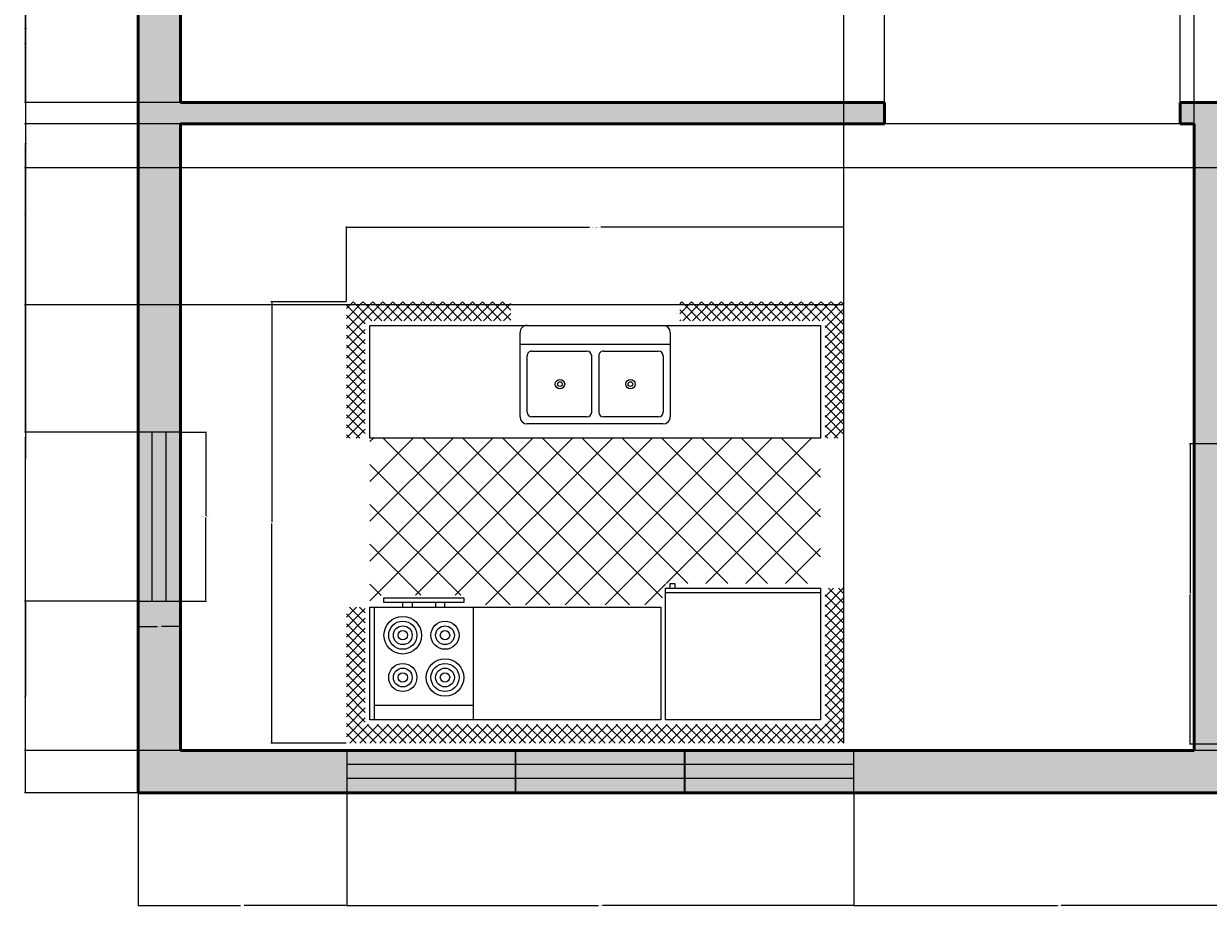
# Model space of a CAD drawing. Units: inches. Extents: x 1201 to 1754, y 247 to 775.
# Tile 1 of 10: x 1222 to 1475, y 247 to 435. Entities that reach past the tile are written whole.
import ezdxf

# ---------------------------------------------------------------- set-up
doc = ezdxf.new("R2010")
doc.units = ezdxf.units.IN
for name, color, linetype, lineweight in [('A-ANNO-DIMS', 2, 'Continuous', 18), ('A-FLOR-FIXT', 8, 'Continuous', 20), ('A-GLAZ', 4, 'Continuous', 18), ('A-GLAZ-PATT', 9, 'Continuous', 13), ('A-WALL', 7, 'Continuous', 50), ('A-WALL-PATT', 9, 'Continuous', 13)]:
    doc.layers.add(name, color=color, linetype=linetype, lineweight=lineweight)
doc.styles.get("Standard").update_dxf_attribs({"font": 'arial.ttf'})
doc.dimstyles.get("Standard").update_dxf_attribs({"dimtxt": 0.18, "dimasz": 0.18, "dimexe": 0.18, "dimexo": 0.0625, "dimgap": 0.09, "dimtad": 0, "dimtih": 1, "dimtoh": 1, "dimdec": 4, "dimzin": 0, "dimdsep": 46, "dimtxsty": 'Standard', "dimcen": 0.09, "dimadec": 0, "dimazin": 0, "dimtfac": 1, "dimtdec": 4, "dimtofl": 0, "dimtmove": 0, "dimatfit": 3, "dimfxl": 1, "dimtolj": 1, "dimtzin": 0, "dimarcsym": 0})

# ---------------------------------------------------------------- blocks, each defined once
blk = doc.blocks.new('Kitchen Layout - 7 x 8 ft')
for p, q in [((-5, 81.32), (2.68, 89)), ((-5, 83.44), (0.56, 89)), ((-5, 85.56), (-1.56, 89)), ((-5, 87.68), (-3.68, 89)), ((-1, 84.97), (-5, 88.97)), ((1.09, 85), (-2.91, 89)), ((3.21, 85), (-0.79, 89)), ((0.81, 85), (4.81, 89)), ((5.34, 85), (1.34, 89)), ((2.93, 85), (6.93, 89)), ((7.46, 85), (3.46, 89)), ((5.05, 85), (9.05, 89)), ((9.58, 85), (5.58, 89)), ((7.17, 85), (11.17, 89)), ((11.7, 85), (7.7, 89)), ((9.29, 85), (13.29, 89)), ((13.82, 85), (9.82, 89)), ((11.41, 85), (15.41, 89)), ((15.94, 85), (11.94, 89)), ((13.53, 85), (17.53, 89)), ((18.06, 85), (14.06, 89)), ((15.65, 85), (19.65, 89)), ((20.18, 85), (16.18, 89)), ((17.78, 85), (21.78, 89)), ((22.31, 85), (18.31, 89)), ((19.9, 85), (23.9, 89)), ((24.43, 85), (20.43, 89)), ((22.02, 85), (26.02, 89)), ((26.55, 85), (22.55, 89)), ((24.14, 85), (28.14, 89)), ((28.67, 85), (24.67, 89)), ((26.26, 85), (30.26, 89)), ((30.79, 85), (26.79, 89)), ((28.38, 85), (32.38, 89)), ((32.91, 85), (28.91, 89)), ((30.5, 85), (34.5, 89)), ((35.03, 85), (31.03, 89)), ((32.63, 85), (36.63, 89)), ((37.16, 85), (33.16, 89)), ((34.75, 85), (38.75, 89)), ((39.28, 85), (35.28, 89)), ((36.87, 85), (40.87, 89)), ((41.4, 85), (37.4, 89)), ((38.99, 85), (42.99, 89)), ((43.52, 85), (39.52, 89)), ((41.11, 85), (45.11, 89)), ((45.64, 85), (41.64, 89)), ((43.23, 85), (47.23, 89)), ((47.76, 85), (43.76, 89)), ((45.35, 85), (49.35, 89)), ((49.88, 85), (45.88, 89)), ((47.47, 85), (51.47, 89)), ((52, 85), (48, 89)), ((49.6, 85), (53.6, 89)), ((54.13, 85), (50.13, 89)), ((51.72, 85), (55.72, 89)), ((56.25, 85), (52.25, 89)), ((53.84, 85), (57.84, 89)), ((58.37, 85), (54.37, 89)), ((55.96, 85), (59.96, 89)), ((60.49, 85), (56.49, 89)), ((58.08, 85), (62.08, 89)), ((62.61, 85), (58.61, 89)), ((60.2, 85), (64.2, 89)), ((64.73, 85), (60.73, 89)), ((62.32, 85), (66.32, 89)), ((66.85, 85), (62.85, 89)), ((64.45, 85), (68.45, 89)), ((68.97, 85), (64.97, 89)), ((66.57, 85), (70.57, 89)), ((71.1, 85), (67.1, 89)), ((68.69, 85), (72.69, 89)), ((73.22, 85), (69.22, 89)), ((70.81, 85), (74.81, 89)), ((75.34, 85), (71.34, 89)), ((72.93, 85), (76.93, 89)), ((77.46, 85), (73.46, 89)), ((75.05, 85), (79.05, 89)), ((79.58, 85), (75.58, 89)), ((77.17, 85), (81.17, 89)), ((81.7, 85), (77.7, 89)), ((79.29, 85), (83.29, 89)), ((83.82, 85), (79.82, 89)), ((81.42, 85), (85.42, 89)), ((85.95, 85), (81.95, 89)), ((83.54, 85), (87.54, 89)), ((88.07, 85), (84.07, 89)), ((85.66, 85), (89.66, 89)), ((90.19, 85), (86.19, 89)), ((87.78, 85), (91.78, 89)), ((92.31, 85), (88.31, 89)), ((89.9, 85), (93.9, 89)), ((94.43, 85), (90.43, 89)), ((92.02, 85), (96.02, 89)), ((96.55, 85), (92.55, 89)), ((94.14, 85), (98.14, 89)), ((101, 82.67), (94.67, 89)), ((96.27, 85), (100.27, 89)), ((101, 84.79), (96.79, 89)), ((101, 86.92), (98.92, 89)), ((-1, 82.85), (-5, 86.85)), ((97, 83.61), (101, 87.61)), ((-1, 80.73), (-5, 84.73)), ((34, 84), (96, 84)), ((34, 60), (34, 84)), ((96, 84), (96, 60)), ((97, 81.49), (101, 85.49)), ((101, 80.55), (97, 84.55)), ((97, 79.37), (101, 83.37)), ((-5, 79.19), (-1, 83.19)), ((-1, 78.61), (-5, 82.61)), ((-5, 77.07), (-1, 81.07)), ((74, 81), (95, 81)), ((101, 78.43), (97, 82.43)), ((97, 77.25), (101, 81.25)), ((-1, 76.49), (-5, 80.49)), ((-5, 74.95), (-1, 78.95)), ((-1, 74.36), (-5, 78.36)), ((101, 76.31), (97, 80.31)), ((97, 75.13), (101, 79.13)), ((-5, 72.83), (-1, 76.83)), ((-1, 72.24), (-5, 76.24)), ((101, 74.19), (97, 78.19)), ((97, 73.01), (101, 77.01)), ((101, 72.07), (97, 76.07)), ((-5, 70.71), (-1, 74.71)), ((-1, 70.12), (-5, 74.12)), ((97, 70.89), (101, 74.89)), ((101, 69.95), (97, 73.95)), ((-5, 68.59), (-1, 72.59)), ((-1, 68), (-5, 72)), ((97, 68.76), (101, 72.76)), ((101, 67.82), (97, 71.82)), ((-5, 66.47), (-1, 70.47)), ((-1, 65.88), (-5, 69.88)), ((-5, 64.35), (-1, 68.35)), ((97, 66.64), (101, 70.64)), ((101, 65.7), (97, 69.7)), ((97, 64.52), (101, 68.52)), ((-1, 63.76), (-5, 67.76)), ((-5, 62.22), (-1, 66.22)), ((-1, 61.64), (-5, 65.64)), ((101, 63.58), (97, 67.58)), ((97, 62.4), (101, 66.4)), ((-5, 60.1), (-1, 64.1)), ((-1, 59.52), (-5, 63.52)), ((101, 61.46), (97, 65.46)), ((97, 60.28), (101, 64.28)), ((100.34, 60), (97, 63.34)), ((-5, 57.98), (-1, 61.98)), ((-1, 57.39), (-5, 61.39)), ((98.22, 60), (97, 61.22)), ((98.84, 60), (101, 62.16)), ((-1.73, 56), (-5, 59.27)), ((-4.86, 56), (-1, 59.86)), ((10.4, 24), (45.9, 59.5)), ((18.88, 24), (54.38, 59.5)), ((27.37, 24), (62.87, 59.5)), ((33.03, 55.11), (37.41, 59.5)), ((96, 60), (34, 60)), ((35.85, 24), (71.35, 59.5)), ((76.2, 24), (40.7, 59.5)), ((84.68, 24), (49.18, 59.5)), ((93.17, 24), (57.67, 59.5)), ((61.31, 24), (96, 58.69)), ((96, 29.65), (66.15, 59.5)), ((80, 60), (80, 59)), ((82, 59), (82, 60)), ((87, 59), (87, 60)), ((89, 60), (89, 59)), ((100.96, 60), (101, 60.04)), ((-3.85, 56), (-5, 57.15)), ((-2.74, 56), (-1, 57.74)), ((0, 57), (33, 57)), ((31, 55), (31, 56)), ((32, 56), (32, 55)), ((67.71, 24), (33.68, 58.04)), ((44.34, 24), (77.84, 57.5)), ((52.82, 24), (86.32, 57.5)), ((96, 38.14), (76.64, 57.5)), ((96, 46.63), (85.13, 57.5)), ((96, 55.11), (93.57, 57.54)), ((0, 30.57), (24.43, 55)), ((0, 39.06), (15.94, 55)), ((0, 47.54), (7.46, 55)), ((1.91, 24), (32.91, 55)), ((33.77, 24), (2.77, 55)), ((42.26, 24), (11.26, 55)), ((50.74, 24), (19.74, 55)), ((59.23, 24), (28.23, 55)), ((32, 55), (31, 55)), ((25.29, 24), (0, 49.29)), ((69.79, 24), (96, 50.21)), ((16.8, 24), (0, 40.8)), ((78.28, 24), (96, 41.72)), ((86.76, 24), (96, 33.24)), ((8.32, 24), (0, 32.32)), ((-5, 21.92), (-2.92, 24)), ((-5, 19.8), (-1, 23.8)), ((-1, 19.21), (-5, 23.21)), ((-1, 21.33), (-3.67, 24)), ((-1, 23.45), (-1.55, 24)), ((0, 24), (96, 24)), ((0, 0), (0, 24)), ((95.25, 24), (96, 24.75)), ((96, 24), (96, 0)), ((97, 22.1), (98.9, 24)), ((97, 19.97), (101, 23.97)), ((101, 19.03), (97, 23.03)), ((101, 21.16), (98.16, 24)), ((101, 23.28), (100.28, 24)), ((-5, 17.68), (-1, 21.68)), ((-1, 17.09), (-5, 21.09)), ((97, 17.85), (101, 21.85)), ((101, 16.91), (97, 20.91)), ((-5, 15.55), (-1, 19.55)), ((-1, 14.97), (-5, 18.97)), ((47.25, 6.5), (47.25, 18.5)), ((48.75, 18.5), (48.75, 6.5)), ((97, 15.73), (101, 19.73)), ((101, 14.79), (97, 18.79)), ((-5, 13.43), (-1, 17.43)), ((-1, 12.85), (-5, 16.85)), ((-5, 11.31), (-1, 15.31)), ((97, 13.61), (101, 17.61)), ((101, 12.67), (97, 16.67)), ((97, 11.49), (101, 15.49)), ((-1, 10.73), (-5, 14.73)), ((-5, 9.19), (-1, 13.19)), ((101, 10.55), (97, 14.55)), ((97, 9.37), (101, 13.37)), ((-1, 8.6), (-5, 12.6)), ((-5, 7.07), (-1, 11.07)), ((-1, 6.48), (-5, 10.48)), ((101, 8.43), (97, 12.43)), ((97, 7.25), (101, 11.25)), ((101, 6.31), (97, 10.31)), ((-5, 4.95), (-1, 8.95)), ((-1, 4.36), (-5, 8.36)), ((97, 5.12), (101, 9.12)), ((101, 4.18), (97, 8.18)), ((-5, 2.83), (-1, 6.83)), ((-1, 2.24), (-5, 6.24)), ((97, 3), (101, 7)), ((101, 2.06), (97, 6.06)), ((-5, 0.71), (-1, 4.71)), ((-1, 0.12), (-5, 4.12)), ((-5, -1.42), (-1, 2.58)), ((64, 4), (32, 4)), ((93.24, -5), (101, 2.76)), ((97, 0.88), (101, 4.88)), ((101, -0.06), (97, 3.94)), ((2, -5), (-5, 2)), ((-5, -3.54), (-1, 0.46)), ((96, 0), (0, 0)), ((95.36, -5), (101, 0.64)), ((101, -2.18), (97, 1.82)), ((-0.12, -5), (-5, -0.12)), ((-2.25, -5), (-5, -2.25)), ((-4.34, -5), (-0.34, -1)), ((-2.22, -5), (1.78, -1)), ((-0.1, -5), (3.9, -1)), ((4.12, -5), (0.12, -1)), ((2.02, -5), (6.02, -1)), ((6.24, -5), (2.24, -1)), ((4.14, -5), (8.14, -1)), ((8.36, -5), (4.36, -1)), ((6.27, -5), (10.27, -1)), ((10.48, -5), (6.48, -1)), ((8.39, -5), (12.39, -1)), ((12.6, -5), (8.6, -1)), ((10.51, -5), (14.51, -1)), ((14.73, -5), (10.73, -1)), ((12.63, -5), (16.63, -1)), ((16.85, -5), (12.85, -1)), ((14.75, -5), (18.75, -1)), ((18.97, -5), (14.97, -1)), ((16.87, -5), (20.87, -1)), ((21.09, -5), (17.09, -1)), ((18.99, -5), (22.99, -1)), ((23.21, -5), (19.21, -1)), ((21.11, -5), (25.11, -1)), ((25.33, -5), (21.33, -1)), ((23.24, -5), (27.24, -1)), ((27.45, -5), (23.45, -1)), ((25.36, -5), (29.36, -1)), ((29.57, -5), (25.57, -1)), ((27.48, -5), (30, -2.48)), ((30, -3.3), (27.7, -1)), ((30, -1.18), (29.82, -1)), ((66, -2.54), (67.54, -1)), ((66, -4.66), (69.66, -1)), ((69.88, -5), (66, -1.12)), ((67.78, -5), (71.78, -1)), ((72, -5), (68, -1)), ((69.9, -5), (73.9, -1)), ((74.12, -5), (70.12, -1)), ((72.03, -5), (76.03, -1)), ((76.24, -5), (72.24, -1)), ((74.15, -5), (78.15, -1)), ((78.36, -5), (74.36, -1)), ((76.27, -5), (80.27, -1)), ((80.49, -5), (76.49, -1)), ((78.39, -5), (82.39, -1)), ((82.61, -5), (78.61, -1)), ((80.51, -5), (84.51, -1)), ((84.73, -5), (80.73, -1)), ((82.63, -5), (86.63, -1)), ((86.85, -5), (82.85, -1)), ((84.75, -5), (88.75, -1)), ((88.97, -5), (84.97, -1)), ((86.88, -5), (90.88, -1)), ((91.09, -5), (87.09, -1)), ((89, -5), (93, -1)), ((93.21, -5), (89.21, -1)), ((91.12, -5), (95.12, -1)), ((95.34, -5), (91.34, -1)), ((97.46, -5), (93.46, -1)), ((99.58, -5), (95.58, -1)), ((101, -4.3), (97, -0.3)), ((97.48, -5), (101, -1.48)), ((-4.37, -5), (-5, -4.37)), ((29.6, -5), (30, -4.6)), ((67.76, -5), (66, -3.24)), ((99.6, -5), (101, -3.6))]:
    blk.add_line(p, q)
for points in [[(0, 56), (0, 84), (33, 84), (33, 56)], [(74, 60), (74, 84), (95, 84), (95, 60)], [(76, 58), (76, 59), (93, 59), (93, 58)]]:
    blk.add_lwpolyline(points, close=True)
for points in [[(33.5, 21), (62.5, 21)], [(32, 1.5), (32, 19.5)], [(33.5, 6.5), (33.5, 18.5)], [(34.5, 19.5), (46.25, 19.5)], [(49.75, 19.5), (61.5, 19.5)], [(62.5, 18.5), (62.5, 6.5)], [(64, 19.5), (64, 1.5)], [(46.25, 5.5), (34.5, 5.5)], [(61.5, 5.5), (49.75, 5.5)], [(62.5, 0), (33.5, 0)]]:
    blk.add_lwpolyline(points)
for centre, radius in [((80, 75), 4), ((80, 75), 3), ((80, 75), 2), ((80, 75), 1), ((89, 75), 3), ((89, 75), 2), ((89, 75), 1), ((80, 66), 3), ((89, 66), 4), ((89, 66), 3), ((80, 66), 2), ((80, 66), 1), ((89, 66), 2), ((89, 66), 1), ((40.5, 12.5), 1), ((40.5, 12.5), 0.5), ((55.5, 12.5), 1), ((55.5, 12.5), 0.5)]:
    blk.add_circle(centre, radius)
for centre, radius, start, end in [((33.5, 19.5), 1.5, 90, 180), ((62.5, 19.5), 1.5, 0, 90), ((34.5, 18.5), 1, 90, 180), ((46.25, 18.5), 1, 0, 90), ((49.75, 18.5), 1, 90, 180), ((61.5, 18.5), 1, 0, 90), ((34.5, 6.5), 1, 180, 270), ((46.25, 6.5), 1, 270, 0), ((49.75, 6.5), 1, 180, 270), ((61.5, 6.5), 1, 270, 0), ((33.5, 1.5), 1.5, 180, 270), ((62.5, 1.5), 1.5, 270, 0)]:
    blk.add_arc(centre, radius, start, end)
blk = doc.blocks.new('WIN-36IN-PLAN')
for p, q in [((9, 36), (0, 36)), ((3, 0), (3, 36)), ((6, 0), (6, 36))]:
    blk.add_line(p, q)
blk.add_lwpolyline([(0, 36), (0, 0), (9, 0), (9, 36)])
blk = doc.blocks.new('*D19')
at = {"layer": 'A-ANNO-DIMS', "color": 0, "lineweight": -2, "transparency": 16777216}
for p, q in [((1255.58, 347.75), (1261.1, 347.75)), ((1260.92, 347.57), (1260.92, 329.93)), ((1260.92, 311.93), (1260.92, 329.57)), ((1255.58, 311.75), (1261.1, 311.75))]:
    blk.add_line(p, q, dxfattribs=at)
at = {"layer": 'A-ANNO-DIMS', "color": 0, "transparency": 16777216}
for points in [[(1260.89, 347.57), (1260.95, 347.57), (1260.92, 347.75)], [(1260.89, 311.93), (1260.95, 311.93), (1260.92, 311.75)]]:
    blk.add_solid(points, dxfattribs=at)
at = {"layer": 'Defpoints', "color": 0, "transparency": 16777216}
for p in [(1255.52, 347.75), (1260.92, 347.75), (1255.52, 311.75)]:
    blk.add_point(p, dxfattribs=at)
at = {"layer": 'A-ANNO-DIMS', "color": 0, "transparency": 16777216, "insert": (1260.92, 329.75), "char_height": 0.18, "attachment_point": 5}
blk.add_mtext('\\A1;WINDOW 36 TYP.', dxfattribs=at)
blk = doc.blocks.new('*D20')
at = {"layer": 'A-ANNO-DIMS', "color": 0, "lineweight": -2, "transparency": 16777216}
for p, q in [((1246.52, 311.69), (1246.52, 306.17)), ((1255.52, 311.69), (1255.52, 306.17)), ((1246.7, 306.35), (1250.56, 306.35)), ((1255.34, 306.35), (1251.48, 306.35))]:
    blk.add_line(p, q, dxfattribs=at)
at = {"layer": 'A-ANNO-DIMS', "color": 0, "transparency": 16777216}
for points in [[(1246.7, 306.38), (1246.7, 306.32), (1246.52, 306.35)], [(1255.34, 306.38), (1255.34, 306.32), (1255.52, 306.35)]]:
    blk.add_solid(points, dxfattribs=at)
at = {"layer": 'Defpoints', "color": 0, "transparency": 16777216}
for p in [(1246.52, 311.75), (1255.52, 311.75), (1255.52, 306.35)]:
    blk.add_point(p, dxfattribs=at)
at = {"layer": 'A-ANNO-DIMS', "color": 0, "transparency": 16777216, "insert": (1251.02, 306.35), "char_height": 0.18, "attachment_point": 5}
blk.add_mtext('\\A1;9 TYP.', dxfattribs=at)
blk = doc.blocks.new('*D39')
at = {"layer": 'A-ANNO-DIMS', "color": 0, "lineweight": -2, "transparency": 16777216}
for p, q in [((1290.89, 375.55), (1290.89, 391.57)), ((1291.07, 391.39), (1342.69, 391.39)), ((1396.71, 391.39), (1345.09, 391.39)), ((1396.89, 375.55), (1396.89, 391.57))]:
    blk.add_line(p, q, dxfattribs=at)
at = {"layer": 'A-ANNO-DIMS', "color": 0, "transparency": 16777216}
for points in [[(1291.07, 391.42), (1291.07, 391.36), (1290.89, 391.39)], [(1396.71, 391.42), (1396.71, 391.36), (1396.89, 391.39)]]:
    blk.add_solid(points, dxfattribs=at)
at = {"layer": 'Defpoints', "color": 0, "transparency": 16777216}
for p in [(1290.89, 391.39), (1290.89, 375.49), (1396.89, 375.49)]:
    blk.add_point(p, dxfattribs=at)
at = {"layer": 'A-ANNO-DIMS', "color": 0, "transparency": 16777216, "insert": (1343.89, 391.39), "char_height": 0.18, "attachment_point": 5}
blk.add_mtext('\\A1;KITCHEN UNIT 106', dxfattribs=at)
blk = doc.blocks.new('*D40')
at = {"layer": 'A-ANNO-DIMS', "color": 0, "lineweight": -2, "transparency": 16777216}
for p, q in [((1290.83, 375.49), (1274.81, 375.49)), ((1274.99, 375.31), (1274.99, 328.67)), ((1274.99, 281.67), (1274.99, 328.31)), ((1290.83, 281.49), (1274.81, 281.49))]:
    blk.add_line(p, q, dxfattribs=at)
at = {"layer": 'A-ANNO-DIMS', "color": 0, "transparency": 16777216}
for points in [[(1274.96, 375.31), (1275.02, 375.31), (1274.99, 375.49)], [(1274.96, 281.67), (1275.02, 281.67), (1274.99, 281.49)]]:
    blk.add_solid(points, dxfattribs=at)
at = {"layer": 'Defpoints', "color": 0, "transparency": 16777216}
for p in [(1290.89, 375.49), (1274.99, 281.49), (1290.89, 281.49)]:
    blk.add_point(p, dxfattribs=at)
at = {"layer": 'A-ANNO-DIMS', "color": 0, "transparency": 16777216, "insert": (1274.99, 328.49), "char_height": 0.18, "attachment_point": 5}
blk.add_mtext('\\A1;94', dxfattribs=at)
blk = doc.blocks.new('*D43')
at = {"layer": 'A-ANNO-DIMS', "color": 0, "lineweight": -2, "transparency": 16777216}
for p, q in [((1480.23, 345.28), (1470.51, 345.28)), ((1470.69, 345.1), (1470.69, 313.47)), ((1470.69, 281.46), (1470.69, 313.1)), ((1480.23, 281.28), (1470.51, 281.28))]:
    blk.add_line(p, q, dxfattribs=at)
at = {"layer": 'A-ANNO-DIMS', "color": 0, "transparency": 16777216}
for points in [[(1470.66, 345.1), (1470.72, 345.1), (1470.69, 345.28)], [(1470.66, 281.46), (1470.72, 281.46), (1470.69, 281.28)]]:
    blk.add_solid(points, dxfattribs=at)
at = {"layer": 'Defpoints', "color": 0, "transparency": 16777216}
for p in [(1480.29, 345.28), (1470.69, 281.28), (1480.29, 281.28)]:
    blk.add_point(p, dxfattribs=at)
at = {"layer": 'A-ANNO-DIMS', "color": 0, "transparency": 16777216, "insert": (1470.69, 313.28), "char_height": 0.18, "attachment_point": 5}
blk.add_mtext('\\A1;REFRIGERATOR 64', dxfattribs=at)
blk = doc.blocks.new('*D50')
at = {"layer": 'A-ANNO-DIMS', "color": 0, "lineweight": -2, "transparency": 16777216}
for p, q in [((1255.46, 557.44), (1222.33, 557.44)), ((1222.51, 557.26), (1222.51, 487.87)), ((1222.51, 418.12), (1222.51, 487.51)), ((1255.46, 417.94), (1222.33, 417.94))]:
    blk.add_line(p, q, dxfattribs=at)
at = {"layer": 'A-ANNO-DIMS', "color": 0, "transparency": 16777216}
for points in [[(1222.48, 557.26), (1222.54, 557.26), (1222.51, 557.44)], [(1222.48, 418.12), (1222.54, 418.12), (1222.51, 417.94)]]:
    blk.add_solid(points, dxfattribs=at)
at = {"layer": 'Defpoints', "color": 0, "transparency": 16777216}
for p in [(1255.52, 557.44), (1222.51, 417.94), (1255.52, 417.94)]:
    blk.add_point(p, dxfattribs=at)
at = {"layer": 'A-ANNO-DIMS', "color": 0, "transparency": 16777216, "insert": (1222.51, 487.69), "char_height": 0.18, "attachment_point": 5}
blk.add_mtext('\\A1;139.5', dxfattribs=at)
blk = doc.blocks.new('*D51')
at = {"layer": 'A-ANNO-DIMS', "color": 0, "lineweight": -2, "transparency": 16777216}
for p, q in [((1471.46, 413.44), (1222.33, 413.44)), ((1222.51, 413.26), (1222.51, 346.87)), ((1222.51, 280.12), (1222.51, 346.51)), ((1471.46, 279.94), (1222.33, 279.94))]:
    blk.add_line(p, q, dxfattribs=at)
at = {"layer": 'A-ANNO-DIMS', "color": 0, "transparency": 16777216}
for points in [[(1222.48, 413.26), (1222.54, 413.26), (1222.51, 413.44)], [(1222.48, 280.12), (1222.54, 280.12), (1222.51, 279.94)]]:
    blk.add_solid(points, dxfattribs=at)
at = {"layer": 'Defpoints', "color": 0, "transparency": 16777216}
for p in [(1471.52, 413.44), (1222.51, 279.94), (1471.52, 279.94)]:
    blk.add_point(p, dxfattribs=at)
at = {"layer": 'A-ANNO-DIMS', "color": 0, "transparency": 16777216, "insert": (1222.51, 346.69), "char_height": 0.18, "attachment_point": 5}
blk.add_mtext('\\A1;133.5', dxfattribs=at)
blk = doc.blocks.new('*D58')
at = {"layer": 'A-ANNO-DIMS', "color": 0, "lineweight": -2, "transparency": 16777216}
for p, q in [((1405.52, 418), (1405.52, 775.14)), ((1405.7, 774.96), (1436.8, 774.96)), ((1468.34, 774.96), (1437.24, 774.96)), ((1468.52, 418), (1468.52, 775.14))]:
    blk.add_line(p, q, dxfattribs=at)
at = {"layer": 'A-ANNO-DIMS', "color": 0, "transparency": 16777216}
for points in [[(1405.7, 774.99), (1405.7, 774.93), (1405.52, 774.96)], [(1468.34, 774.99), (1468.34, 774.93), (1468.52, 774.96)]]:
    blk.add_solid(points, dxfattribs=at)
at = {"layer": 'Defpoints', "color": 0, "transparency": 16777216}
for p in [(1468.52, 774.96), (1405.52, 417.94), (1468.52, 417.94)]:
    blk.add_point(p, dxfattribs=at)
at = {"layer": 'A-ANNO-DIMS', "color": 0, "transparency": 16777216, "insert": (1437.02, 774.96), "char_height": 0.18, "attachment_point": 5}
blk.add_mtext('\\A1;63', dxfattribs=at)
blk = doc.blocks.new('*D59')
at = {"layer": 'A-ANNO-DIMS', "color": 0, "lineweight": -2, "transparency": 16777216}
for p, q in [((1255.52, 418), (1255.52, 775.14)), ((1255.7, 774.96), (1330.24, 774.96)), ((1405.34, 774.96), (1330.8, 774.96)), ((1405.52, 418), (1405.52, 775.14))]:
    blk.add_line(p, q, dxfattribs=at)
at = {"layer": 'A-ANNO-DIMS', "color": 0, "transparency": 16777216}
for points in [[(1255.7, 774.99), (1255.7, 774.93), (1255.52, 774.96)], [(1405.34, 774.99), (1405.34, 774.93), (1405.52, 774.96)]]:
    blk.add_solid(points, dxfattribs=at)
at = {"layer": 'Defpoints', "color": 0, "transparency": 16777216}
for p in [(1405.52, 774.96), (1255.52, 417.94), (1405.52, 417.94)]:
    blk.add_point(p, dxfattribs=at)
at = {"layer": 'A-ANNO-DIMS', "color": 0, "transparency": 16777216, "insert": (1330.52, 774.96), "char_height": 0.18, "attachment_point": 5}
blk.add_mtext('\\A1;150', dxfattribs=at)
blk = doc.blocks.new('*D69')
at = {"layer": 'A-ANNO-DIMS', "color": 0, "lineweight": -2, "transparency": 16777216}
for p, q in [((1246.46, 311.75), (1222.33, 311.75)), ((1222.51, 311.57), (1222.51, 291.53)), ((1222.51, 271.12), (1222.51, 291.16)), ((1246.46, 270.94), (1222.33, 270.94))]:
    blk.add_line(p, q, dxfattribs=at)
at = {"layer": 'A-ANNO-DIMS', "color": 0, "transparency": 16777216}
for points in [[(1222.48, 311.57), (1222.54, 311.57), (1222.51, 311.75)], [(1222.48, 271.12), (1222.54, 271.12), (1222.51, 270.94)]]:
    blk.add_solid(points, dxfattribs=at)
at = {"layer": 'Defpoints', "color": 0, "transparency": 16777216}
for p in [(1222.51, 311.75), (1246.52, 311.75), (1246.52, 270.94)]:
    blk.add_point(p, dxfattribs=at)
at = {"layer": 'A-ANNO-DIMS', "color": 0, "transparency": 16777216, "insert": (1222.51, 291.35), "char_height": 0.18, "attachment_point": 5}
blk.add_mtext('\\A1;40.81', dxfattribs=at)
blk = doc.blocks.new('*D70')
at = {"layer": 'A-ANNO-DIMS', "color": 0, "lineweight": -2, "transparency": 16777216}
for p, q in [((1246.46, 470.7), (1222.33, 470.7)), ((1222.51, 470.52), (1222.51, 409.4)), ((1222.51, 347.93), (1222.51, 409.04)), ((1246.46, 347.75), (1222.33, 347.75))]:
    blk.add_line(p, q, dxfattribs=at)
at = {"layer": 'A-ANNO-DIMS', "color": 0, "transparency": 16777216}
for points in [[(1222.48, 470.52), (1222.54, 470.52), (1222.51, 470.7)], [(1222.48, 347.93), (1222.54, 347.93), (1222.51, 347.75)]]:
    blk.add_solid(points, dxfattribs=at)
at = {"layer": 'Defpoints', "color": 0, "transparency": 16777216}
for p in [(1222.51, 470.7), (1246.52, 470.7), (1246.52, 347.75)]:
    blk.add_point(p, dxfattribs=at)
at = {"layer": 'A-ANNO-DIMS', "color": 0, "transparency": 16777216, "insert": (1222.51, 409.22), "char_height": 0.18, "attachment_point": 5}
blk.add_mtext('\\A1;122.95', dxfattribs=at)
blk = doc.blocks.new('*D74')
at = {"layer": 'A-ANNO-DIMS', "color": 0, "lineweight": -2, "transparency": 16777216}
for p, q in [((1717.46, 404.03), (1222.33, 404.03)), ((1222.51, 403.85), (1222.51, 342.17)), ((1222.51, 280.12), (1222.51, 341.81)), ((1717.46, 279.94), (1222.33, 279.94))]:
    blk.add_line(p, q, dxfattribs=at)
at = {"layer": 'A-ANNO-DIMS', "color": 0, "transparency": 16777216}
for points in [[(1222.48, 403.85), (1222.54, 403.85), (1222.51, 404.03)], [(1222.48, 280.12), (1222.54, 280.12), (1222.51, 279.94)]]:
    blk.add_solid(points, dxfattribs=at)
at = {"layer": 'Defpoints', "color": 0, "transparency": 16777216}
for p in [(1222.51, 404.03), (1717.52, 404.03), (1717.52, 279.94)]:
    blk.add_point(p, dxfattribs=at)
at = {"layer": 'A-ANNO-DIMS', "color": 0, "transparency": 16777216, "insert": (1222.51, 341.99), "char_height": 0.18, "attachment_point": 5}
blk.add_mtext('\\A1;124.1', dxfattribs=at)
blk = doc.blocks.new('*D77')
at = {"layer": 'A-ANNO-DIMS', "color": 0, "lineweight": -2, "transparency": 16777216}
for p, q in [((1246.52, 270.88), (1246.52, 246.75)), ((1290.95, 270.88), (1290.95, 246.75)), ((1246.7, 246.93), (1268.34, 246.93)), ((1290.77, 246.93), (1269.13, 246.93))]:
    blk.add_line(p, q, dxfattribs=at)
at = {"layer": 'A-ANNO-DIMS', "color": 0, "transparency": 16777216}
for points in [[(1246.7, 246.96), (1246.7, 246.9), (1246.52, 246.93)], [(1290.77, 246.96), (1290.77, 246.9), (1290.95, 246.93)]]:
    blk.add_solid(points, dxfattribs=at)
at = {"layer": 'Defpoints', "color": 0, "transparency": 16777216}
for p in [(1246.52, 270.94), (1290.95, 270.94), (1290.95, 246.93)]:
    blk.add_point(p, dxfattribs=at)
at = {"layer": 'A-ANNO-DIMS', "color": 0, "transparency": 16777216, "insert": (1268.73, 246.93), "char_height": 0.18, "attachment_point": 5}
blk.add_mtext('\\A1;44.43', dxfattribs=at)
blk = doc.blocks.new('*D78')
at = {"layer": 'A-ANNO-DIMS', "color": 0, "lineweight": -2, "transparency": 16777216}
for p, q in [((1290.95, 270.88), (1290.95, 246.75)), ((1399.01, 270.88), (1399.01, 246.75)), ((1291.13, 246.93), (1344.52, 246.93)), ((1398.83, 246.93), (1345.43, 246.93))]:
    blk.add_line(p, q, dxfattribs=at)
at = {"layer": 'A-ANNO-DIMS', "color": 0, "transparency": 16777216}
for points in [[(1291.13, 246.96), (1291.13, 246.9), (1290.95, 246.93)], [(1398.83, 246.96), (1398.83, 246.9), (1399.01, 246.93)]]:
    blk.add_solid(points, dxfattribs=at)
at = {"layer": 'Defpoints', "color": 0, "transparency": 16777216}
for p in [(1290.95, 270.94), (1399.01, 270.94), (1399.01, 246.93)]:
    blk.add_point(p, dxfattribs=at)
at = {"layer": 'A-ANNO-DIMS', "color": 0, "transparency": 16777216, "insert": (1344.98, 246.93), "char_height": 0.18, "attachment_point": 5}
blk.add_mtext('\\A1;108.06', dxfattribs=at)
blk = doc.blocks.new('*D79')
at = {"layer": 'A-ANNO-DIMS', "color": 0, "lineweight": -2, "transparency": 16777216}
for p, q in [((1399.01, 270.88), (1399.01, 246.75)), ((1486.59, 270.88), (1486.59, 246.75)), ((1399.19, 246.93), (1442.41, 246.93)), ((1486.41, 246.93), (1443.19, 246.93))]:
    blk.add_line(p, q, dxfattribs=at)
at = {"layer": 'A-ANNO-DIMS', "color": 0, "transparency": 16777216}
for points in [[(1399.19, 246.96), (1399.19, 246.9), (1399.01, 246.93)], [(1486.41, 246.96), (1486.41, 246.9), (1486.59, 246.93)]]:
    blk.add_solid(points, dxfattribs=at)
at = {"layer": 'Defpoints', "color": 0, "transparency": 16777216}
for p in [(1399.01, 270.94), (1486.59, 270.94), (1486.59, 246.93)]:
    blk.add_point(p, dxfattribs=at)
at = {"layer": 'A-ANNO-DIMS', "color": 0, "transparency": 16777216, "insert": (1442.8, 246.93), "char_height": 0.18, "attachment_point": 5}
blk.add_mtext('\\A1;87.58', dxfattribs=at)
blk = doc.blocks.new('*D89')
at = {"layer": 'A-ANNO-DIMS', "color": 0, "lineweight": -2, "transparency": 16777216}
for p, q in [((1396.89, 281.58), (1396.89, 775.14)), ((1397.07, 774.96), (1433.81, 774.96)), ((1471.34, 774.96), (1434.6, 774.96)), ((1471.52, 280), (1471.52, 775.14))]:
    blk.add_line(p, q, dxfattribs=at)
at = {"layer": 'A-ANNO-DIMS', "color": 0, "transparency": 16777216}
for points in [[(1397.07, 774.99), (1397.07, 774.93), (1396.89, 774.96)], [(1471.34, 774.99), (1471.34, 774.93), (1471.52, 774.96)]]:
    blk.add_solid(points, dxfattribs=at)
at = {"layer": 'Defpoints', "color": 0, "transparency": 16777216}
for p in [(1471.52, 774.96), (1396.89, 281.52), (1471.52, 279.94)]:
    blk.add_point(p, dxfattribs=at)
at = {"layer": 'A-ANNO-DIMS', "color": 0, "transparency": 16777216, "insert": (1434.21, 774.96), "char_height": 0.18, "attachment_point": 5}
blk.add_mtext('\\A1;74.63', dxfattribs=at)
blk = doc.blocks.new('*D90')
at = {"layer": 'A-ANNO-DIMS', "color": 0, "lineweight": -2, "transparency": 16777216}
for p, q in [((1405.46, 413.44), (1222.33, 413.44)), ((1222.51, 413.26), (1222.51, 394.33)), ((1222.51, 375.03), (1222.51, 393.97)), ((1396.83, 374.85), (1222.33, 374.85))]:
    blk.add_line(p, q, dxfattribs=at)
at = {"layer": 'A-ANNO-DIMS', "color": 0, "transparency": 16777216}
for points in [[(1222.48, 413.26), (1222.54, 413.26), (1222.51, 413.44)], [(1222.48, 375.03), (1222.54, 375.03), (1222.51, 374.85)]]:
    blk.add_solid(points, dxfattribs=at)
at = {"layer": 'Defpoints', "color": 0, "transparency": 16777216}
for p in [(1222.51, 413.44), (1405.52, 413.44), (1396.89, 374.85)]:
    blk.add_point(p, dxfattribs=at)
at = {"layer": 'A-ANNO-DIMS', "color": 0, "transparency": 16777216, "insert": (1222.51, 394.15), "char_height": 0.18, "attachment_point": 5}
blk.add_mtext('\\A1;38.59', dxfattribs=at)
blk = doc.blocks.new('*D93')
at = {"layer": 'A-ANNO-DIMS', "color": 0, "lineweight": -2, "transparency": 16777216}
for p, q in [((1278.95, 443.23), (1222.33, 443.23)), ((1222.51, 443.05), (1222.51, 430.77)), ((1222.51, 418.12), (1222.51, 430.4)), ((1255.46, 417.94), (1222.33, 417.94))]:
    blk.add_line(p, q, dxfattribs=at)
at = {"layer": 'A-ANNO-DIMS', "color": 0, "transparency": 16777216}
for points in [[(1222.48, 443.05), (1222.54, 443.05), (1222.51, 443.23)], [(1222.48, 418.12), (1222.54, 418.12), (1222.51, 417.94)]]:
    blk.add_solid(points, dxfattribs=at)
at = {"layer": 'Defpoints', "color": 0, "transparency": 16777216}
for p in [(1222.51, 443.23), (1279.02, 443.23), (1255.52, 417.94)]:
    blk.add_point(p, dxfattribs=at)
at = {"layer": 'A-ANNO-DIMS', "color": 0, "transparency": 16777216, "insert": (1222.51, 430.58), "char_height": 0.18, "attachment_point": 5}
blk.add_mtext('\\A1;25.285', dxfattribs=at)
blk = doc.blocks.new('*D95')
at = {"layer": 'A-ANNO-DIMS', "color": 0, "lineweight": -2, "transparency": 16777216}
for p, q in [((1366.15, 449.58), (1222.33, 449.58)), ((1222.51, 449.4), (1222.51, 433.94)), ((1222.51, 418.12), (1222.51, 433.58)), ((1405.46, 417.94), (1222.33, 417.94))]:
    blk.add_line(p, q, dxfattribs=at)
at = {"layer": 'A-ANNO-DIMS', "color": 0, "transparency": 16777216}
for points in [[(1222.48, 449.4), (1222.54, 449.4), (1222.51, 449.58)], [(1222.48, 418.12), (1222.54, 418.12), (1222.51, 417.94)]]:
    blk.add_solid(points, dxfattribs=at)
at = {"layer": 'Defpoints', "color": 0, "transparency": 16777216}
for p in [(1366.21, 449.58), (1222.51, 417.94), (1405.52, 417.94)]:
    blk.add_point(p, dxfattribs=at)
at = {"layer": 'A-ANNO-DIMS', "color": 0, "transparency": 16777216, "insert": (1222.51, 433.76), "char_height": 0.18, "attachment_point": 5}
blk.add_mtext('\\A1;31.64', dxfattribs=at)

msp = doc.modelspace()

# ---------------------------------------------------------------- hatches: boundary and pattern name
at = {"layer": 'A-GLAZ-PATT'}
h = msp.add_hatch(color=256, dxfattribs=at)
h.dxf.hatch_style = 1
h.set_gradient(color1=(0, 0, 255), color2=(255, 255, 0), name='CURVED')
h.paths.add_polyline_path([(1255.5208, 347.7487), (1252.5208, 347.7487), (1252.5208, 311.7487), (1255.5208, 311.7487)])
h.paths.add_polyline_path([(1252.5208, 347.7487), (1249.5208, 347.7487), (1249.5208, 311.7487), (1252.5208, 311.7487)])
h.paths.add_polyline_path([(1249.5208, 347.7487), (1246.5208, 347.7487), (1246.5208, 311.7487), (1249.5208, 311.7487)])
h = msp.add_hatch(color=256, dxfattribs=at)
h.dxf.hatch_style = 1
h.set_gradient(color1=(0, 0, 255), color2=(255, 255, 0), name='SPHERICAL')
h.paths.add_polyline_path([(1326.9481, 279.9415), (1290.9481, 279.9415), (1290.9481, 276.9415), (1326.9481, 276.9415)])
h.paths.add_polyline_path([(1326.9481, 273.9415), (1290.9481, 273.9415), (1290.9481, 270.9415), (1326.9481, 270.9415)])
h.paths.add_polyline_path([(1326.9481, 276.9415), (1290.9481, 276.9415), (1290.9481, 273.9415), (1326.9481, 273.9415)])
h.paths.add_polyline_path([(1362.9481, 279.9415), (1326.9481, 279.9415), (1326.9481, 276.9415), (1362.9481, 276.9415)])
h.paths.add_polyline_path([(1362.9481, 276.9415), (1326.9481, 276.9415), (1326.9481, 273.9415), (1362.9481, 273.9415)])
h.paths.add_polyline_path([(1362.9481, 273.9415), (1326.9481, 273.9415), (1326.9481, 270.9415), (1362.9481, 270.9415)])
h.paths.add_polyline_path([(1399.0105, 276.9415), (1363.0105, 276.9415), (1363.0105, 273.9415), (1399.0105, 273.9415)])
h.paths.add_polyline_path([(1399.0105, 279.9415), (1363.0105, 279.9415), (1363.0105, 276.9415), (1399.0105, 276.9415)])
h.paths.add_polyline_path([(1399.0105, 273.9415), (1363.0105, 273.9415), (1363.0105, 270.9415), (1399.0105, 270.9415)])
at = {"layer": 'A-WALL-PATT'}
h = msp.add_hatch(color=256, dxfattribs=at)
h.dxf.hatch_style = 1
h.paths.add_polyline_path([(1255.5208, 741.9415), (1471.5208, 741.9415), (1471.5208, 684.2327), (1471.5208, 602.9415), (1477.5208, 602.9415), (1477.5208, 669.9415), (1618.5208, 669.9415), (1618.5208, 674.4415), (1477.5208, 674.4415), (1477.5208, 741.9415), (1481.2969, 741.9415), (1481.2969, 750.9415), (1246.5208, 750.9415), (1246.5208, 700.7954), (1255.5208, 700.7954)])
h.paths.add_polyline_path([(1255.5208, 557.4415), (1399.5208, 557.4415), (1399.5208, 617.4415), (1423.5208, 617.4415), (1423.5208, 621.9415), (1392.0208, 621.9415), (1392.0208, 617.4415), (1395.0208, 617.4415), (1395.0208, 561.9415), (1255.5208, 561.9415), (1255.5208, 571.8878), (1246.5208, 571.8878), (1246.5208, 506.6967), (1255.5208, 506.6967)])
h.paths.add_polyline_path([(1255.5208, 664.7954), (1246.5208, 664.7954), (1246.5208, 595.8878), (1255.398, 595.8878), (1255.398, 617.4415), (1315.398, 617.4415), (1356.0208, 617.4415), (1356.0208, 618.0127), (1356.0208, 621.9415), (1255.5208, 621.9415), (1255.5208, 629.6628)])
h.paths.add_polyline_path([(1255.5208, 470.6967), (1246.5208, 470.6967), (1246.5208, 347.7487), (1255.5208, 347.7487), (1255.5208, 413.4415), (1405.5208, 413.4415), (1405.5208, 417.9415), (1255.5208, 417.9415)])
h.paths.add_polyline_path([(1290.9481, 279.9415), (1255.5208, 279.9415), (1255.5208, 311.7487), (1246.5208, 311.7487), (1246.5208, 270.9415), (1290.9481, 270.9415)])
h.paths.add_polyline_path([(1486.5907, 279.9415), (1477.5208, 279.9415), (1477.5208, 417.9415), (1468.5208, 417.9415), (1468.5208, 413.4415), (1471.5208, 413.4415), (1471.5208, 279.9415), (1399.0105, 279.9415), (1399.0105, 270.9415), (1486.5907, 270.9415)])
h.paths.add_polyline_path([(1563.0208, 279.9415), (1542.0208, 279.9415), (1542.0208, 417.9415), (1501.5208, 417.9415), (1501.5208, 413.4415), (1513.81, 413.4415), (1513.8125, 413.6987), (1537.8114, 413.4623), (1537.5208, 383.9637), (1537.5208, 279.9415), (1522.5907, 279.9415), (1522.5907, 270.9415), (1563.0208, 270.9415)])
h.paths.add_polyline_path([(1726.5208, 404.0342), (1717.5208, 404.0342), (1717.5208, 279.9415), (1641.0208, 279.9415), (1641.0208, 270.9415), (1726.5208, 270.9415)])
h.paths.add_polyline_path([(1726.5208, 507.4363), (1717.5208, 507.4363), (1717.5208, 440.0342), (1726.5208, 440.0342)])
h.paths.add_polyline_path([(1726.5208, 611.6009), (1717.5208, 611.6009), (1717.5208, 561.9415), (1477.5208, 561.9415), (1471.5208, 561.9692), (1471.5208, 557.4415), (1717.5208, 557.4415), (1717.5208, 543.4363), (1726.5208, 543.4363)])
h.paths.add_polyline_path([(1726.5208, 750.9415), (1505.2969, 750.9415), (1505.2969, 741.9415), (1697.6884, 741.9415), (1697.6884, 741.9922), (1718.6884, 741.9922), (1718.6884, 733.9922), (1717.5208, 733.9922), (1717.5208, 674.4415), (1660.5208, 674.4415), (1660.5208, 669.9415), (1717.5208, 669.9415), (1717.5208, 647.6009), (1726.5208, 647.6009)])

# ---------------------------------------------------------------- linework, layer by layer
at = {"layer": 'A-WALL'}
for p, q in [((1255.5208, 557.4415), (1255.5208, 417.9415)), ((1405.5208, 417.9415), (1255.5208, 417.9415)), ((1405.5208, 417.9415), (1405.5208, 413.4415)), ((1468.5208, 417.9415), (1468.5208, 413.4415)), ((1477.5208, 417.9415), (1468.5208, 417.9415)), ((1405.5208, 413.4415), (1255.5208, 413.4415)), ((1255.5208, 413.4415), (1255.5208, 279.9415)), ((1471.5208, 413.4415), (1468.5208, 413.4415)), ((1471.5208, 413.4415), (1468.5208, 413.4415)), ((1471.5208, 413.4415), (1471.5208, 279.9415)), ((1255.5208, 279.9415), (1471.5208, 279.9415))]:
    msp.add_line(p, q, dxfattribs=at)
msp.add_lwpolyline([(1638.0208, 270.9415), (1726.5208, 270.9415), (1726.5208, 750.9415), (1246.5208, 750.9415), (1246.5208, 270.9415), (1566.0208, 270.9415)], dxfattribs=at)

# ---------------------------------------------------------------- block references
at = {"layer": 'A-FLOR-FIXT', "rotation": 180}
msp.add_blockref('Kitchen Layout - 7 x 8 ft', (1391.8927, 370.4875), dxfattribs=at)
at = {"layer": 'A-GLAZ'}
msp.add_blockref('WIN-36IN-PLAN', (1246.5208, 311.7487), dxfattribs=at)
for p, rotation in [((1326.9481, 270.9415), 90.00000000000126), ((1362.9481, 270.9415), 90.00000000000126), ((1399.0105, 270.9415), 90.00000000000115)]:
    msp.add_blockref('WIN-36IN-PLAN', p, dxfattribs=dict(at, rotation=rotation))

# ---------------------------------------------------------------- dimensions: what is measured, and where the dimension line sits
at = {"layer": 'A-ANNO-DIMS'}
for base, p1, p2, override, picture, middle in [((1405.5208, 774.9565), (1255.5208, 417.9415), (1405.5208, 417.9415), {"dimdec": 0, "dimlfac": 1, "dimrnd": 0, "dimzin": 0, "dimdsep": 46, "dimlunit": 2}, '*D59', (1330.5208, 774.9565)), ((1471.5208, 774.9565), (1396.8927, 281.5161), (1471.5208, 279.9415), {"dimdec": 2, "dimlfac": 1, "dimrnd": 0, "dimzin": 0, "dimdsep": 46, "dimlunit": 2}, '*D89', (1434.2067, 774.9565)), ((1468.5208, 774.9565), (1405.5208, 417.9415), (1468.5208, 417.9415), {"dimdec": 0, "dimlfac": 1, "dimrnd": 0, "dimzin": 0, "dimdsep": 46, "dimlunit": 2}, '*D58', (1437.0208, 774.9565)), ((1290.9481, 246.9265), (1246.5208, 270.9415), (1290.9481, 270.9415), {"dimdec": 2, "dimlfac": 1, "dimrnd": 0, "dimzin": 0, "dimdsep": 46, "dimlunit": 2}, '*D77', (1268.7345, 246.9265)), ((1399.0105, 246.9265), (1290.9481, 270.9415), (1399.0105, 270.9415), {"dimdec": 2, "dimlfac": 1, "dimrnd": 0, "dimzin": 0, "dimdsep": 46, "dimlunit": 2}, '*D78', (1344.9793, 246.9265)), ((1486.5907, 246.9265), (1399.0105, 270.9415), (1486.5907, 270.9415), {"dimdec": 2, "dimlfac": 1, "dimrnd": 0, "dimzin": 0, "dimdsep": 46, "dimlunit": 2}, '*D79', (1442.8006, 246.9265))]:
    dim = msp.add_linear_dim(base=base, p1=p1, p2=p2, dimstyle='Standard', override=override, dxfattribs=at)
    dim.commit()
    dim.dimension.update_dxf_attribs({"geometry": picture, "text_midpoint": middle})
for base, p1, p2, angle, override, picture, middle in [((1222.5058, 417.9415), (1255.5208, 557.4415), (1255.5208, 417.9415), 90, {"dimdec": 1, "dimlfac": 1, "dimrnd": 0, "dimzin": 0, "dimdsep": 46, "dimlunit": 2}, '*D50', (1222.5058, 487.6915)), ((1222.5058, 470.6967), (1246.5208, 347.7487), (1246.5208, 470.6967), 90, {"dimdec": 2, "dimlfac": 1, "dimrnd": 0, "dimzin": 0, "dimdsep": 46, "dimlunit": 2}, '*D70', (1222.5058, 409.2227)), ((1222.5058, 417.9415), (1366.2113, 449.5839), (1405.5208, 417.9415), 90, {"dimdec": 2, "dimlfac": 1, "dimrnd": 0, "dimzin": 0, "dimdsep": 46, "dimlunit": 2}, '*D95', (1222.5058, 433.7627)), ((1222.5058, 443.2267), (1255.5208, 417.9415), (1279.0165, 443.2267), 90, {"dimdec": 3, "dimlfac": 1, "dimrnd": 0, "dimzin": 0, "dimdsep": 46, "dimlunit": 2}, '*D93', (1222.5058, 430.5841)), ((1222.5058, 279.9415), (1471.5208, 413.4415), (1471.5208, 279.9415), 90, {"dimdec": 1, "dimlfac": 1, "dimrnd": 0, "dimzin": 0, "dimdsep": 46, "dimlunit": 2}, '*D51', (1222.5058, 346.6915)), ((1222.5058, 413.4415), (1396.8927, 374.8542), (1405.5208, 413.4415), 90, {"dimdec": 2, "dimlfac": 1, "dimrnd": 0, "dimzin": 0, "dimdsep": 46, "dimlunit": 2}, '*D90', (1222.5058, 394.1478)), ((1222.5058, 404.0342), (1717.5208, 279.9415), (1717.5208, 404.0342), 90, {"dimdec": 1, "dimlfac": 1, "dimrnd": 0, "dimzin": 0, "dimdsep": 46, "dimlunit": 2}, '*D74', (1222.5058, 341.9878)), ((1274.9927, 281.4875), (1290.8927, 375.4875), (1290.8927, 281.4875), 270, {"dimdec": 0, "dimlfac": 1, "dimrnd": 0, "dimzin": 0, "dimdsep": 46, "dimlunit": 2}, '*D40', (1274.9927, 328.4875)), ((1222.5058, 311.7487), (1246.5208, 270.9415), (1246.5208, 311.7487), 90, {"dimdec": 2, "dimlfac": 1, "dimrnd": 0, "dimzin": 0, "dimdsep": 46, "dimlunit": 2}, '*D69', (1222.5058, 291.3451))]:
    dim = msp.add_linear_dim(base=base, p1=p1, p2=p2, angle=angle, dimstyle='Standard', override=override, dxfattribs=at)
    dim.commit()
    dim.dimension.update_dxf_attribs({"geometry": picture, "text_midpoint": middle})
for base, p1, p2, angle, text, picture, middle in [((1290.8927, 391.3875), (1396.8927, 375.4875), (1290.8927, 375.4875), 180, 'KITCHEN UNIT <>', '*D39', (1343.8927, 391.3875)), ((1260.9208, 347.7487), (1255.5208, 311.7487), (1255.5208, 347.7487), 90, 'WINDOW <> TYP.', '*D19', (1260.9208, 329.7487)), ((1470.6925, 281.284), (1480.2925, 345.284), (1480.2925, 281.284), 270, 'REFRIGERATOR <>', '*D43', (1470.6925, 313.284))]:
    dim = msp.add_linear_dim(base=base, p1=p1, p2=p2, angle=angle, text=text, dimstyle='Standard', override={"dimdec": 0, "dimlfac": 1, "dimrnd": 0, "dimzin": 0, "dimdsep": 46, "dimlunit": 2}, dxfattribs=at)
    dim.commit()
    dim.dimension.update_dxf_attribs({"geometry": picture, "text_midpoint": middle})
dim = msp.add_linear_dim(base=(1255.5208, 306.3487), p1=(1246.5208, 311.7487), p2=(1255.5208, 311.7487), text='<> TYP.', dimstyle='Standard', override={"dimdec": 0, "dimlfac": 1, "dimrnd": 0, "dimzin": 0, "dimdsep": 46, "dimlunit": 2}, dxfattribs=at)
dim.commit()
dim.dimension.update_dxf_attribs({"geometry": '*D20', "text_midpoint": (1251.0208, 306.3487)})

doc.saveas('drawing.dxf')
